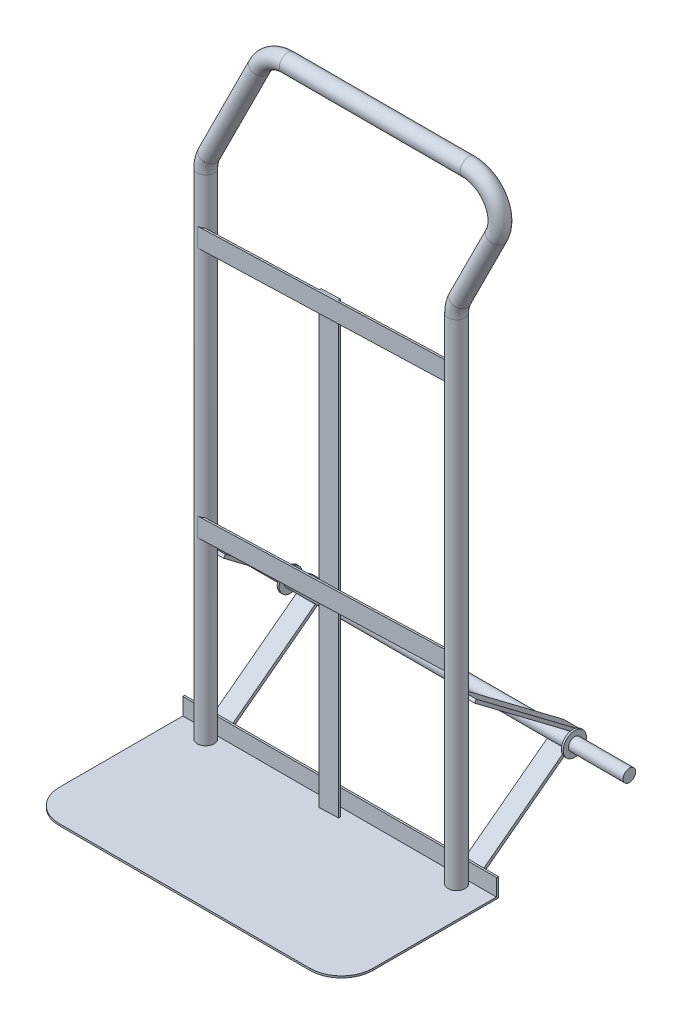
SolidWorks part; units mm, degrees
material "Plain Carbon Steel"
ref_plane "Front Plane" through (0, 0, 0) normal (0, 0, 1) x (1, 0, 0)
ref_plane "Top Plane" through (0, 0, 0) normal (0, 1, 0) x (1, 0, 0)
ref_plane "Right Plane" through (0, 0, 0) normal (1, 0, 0) x (0, 0, -1)
sketch3d "Frame Tube Path 3D Sketch"
  line L0 (0, 0, 0) -> (0, 788.1943, 0)
  line L1 (5.2806, 810.5589, 0) -> (63.8241, 927.6207, 0)
  line L2 (19.1047, 999.9853, 0) -> (-269.0871, 999.9853, 0)
  line L3 (-313.8065, 972.3498, 0) -> (-394.7194, 810.5589, 0)
  line L4 (-400, 788.1943, 0) -> (-400, 0, 0)
  arc A0 (0, 788.1943, 0) -> (5.2806, 810.5589, 0) centre (50, 788.1943, 0) ccw
  arc A1 (63.8241, 927.6207, 0) -> (19.1047, 999.9853, 0) centre (19.1047, 949.9853, 0) ccw
  arc A2 (-269.0871, 999.9853, 0) -> (-313.8065, 972.3498, 0) centre (-269.0871, 949.9853, 0) ccw
  arc A3 (-394.7194, 810.5589, 0) -> (-400, 788.1943, 0) centre (-350, 788.1943, 0) ccw
  point P9 (0, 800, 0)
  point P10 (50, 788.1943, -50)
  point P13 (100.0142, 999.9853, 0)
  point P14 (19.1047, 949.9853, 50)
  point P17 (-299.9858, 999.9853, 0)
  point P18 (-269.0871, 949.9853, 50)
  point P21 (-400, 800, 0)
  point P22 (-350, 788.1943, 50)
  dimension "D8" = 50
  dimension "D1" = 800
  dimension "D2" = 800
  dimension "D3" = 400
  dimension "D4" = 223.6
  dimension "D5" = 223.6
  dimension "D6" = 153.43
  dimension "D7" = 153.43
  dimension "D9" = 63.43
  dimension "D10" = 116.57
other "Pipe 26.9 X 3.2(1)"
ref_plane "Plane1" through (0, 0, 0) normal (0, 1, 0) x (1, 0, 0)
sketch "Sketch1" plane through (0, 0, 0) normal (0, 1, 0) x (1, 0, 0)
  circle A0 centre (0, 0) radius 10.25
  circle A1 centre (0, 0) radius 13.45
  point P3 (0, 13.45)
  point P5 (-13.45, 0)
  point P6 (0, -13.45)
  point P7 (13.45, 0)
  point P8 (0, 0)
  dimension "In_dia" = 20.5
  dimension "Out_dia" = 26.9
ref_plane "Plane2" through (0, 0, 0) normal (0.0336, 0, 0.9994) x (0.9994, 0, -0.0336)
sketch "Cross Bars Sketch" plane through (0, 0, 0) normal (0.0336, 0, 0.9994) x (0.9994, 0, -0.0336)
  line L0 (0, 0) -> (-399.7738, 0) construction
  line L1 (-199.8869, 0) -> (-199.8869, 957.4445) construction
  line L3 (0.1131, 715) -> (-399.8869, 715)
  line L4 (0.1131, 715) -> (0.1131, 685)
  line L5 (0.1131, 685) -> (-399.8869, 685)
  line L6 (-399.8869, 715) -> (-399.8869, 685)
  line L7 (0.1131, 715) -> (-399.8869, 685) construction
  line L8 (0.1131, 685) -> (-399.8869, 715) construction
  line L9 (0.1131, 315) -> (-399.8869, 315)
  line L10 (0.1131, 315) -> (0.1131, 285)
  line L11 (0.1131, 285) -> (-399.8869, 285)
  line L12 (-399.8869, 315) -> (-399.8869, 285)
  line L13 (0.1131, 315) -> (-399.8869, 285) construction
  line L14 (0.1131, 285) -> (-399.8869, 315) construction
  point P6 (-199.8869, 700)
  point P11 (-199.8869, 300)
  dimension "D1" = 30
  dimension "D2" = 400
  dimension "D3" = 30
  dimension "D4" = 400
  dimension "D5" = 370
  dimension "D6" = 715
extrude "Cross Bars 30x3" add sketch "Cross Bars Sketch" against normal blind 3 separate body
sketch "Centre Upright Sketch" plane through (-0.1009, 0, -2.9983) normal (-0.0336, 0, -0.9994) x (-0.9994, 0, 0.0336)
  line L0 (199.8869, 0) -> (199.8869, 715) construction
  line L2 (-0.1131, 315) -> (399.8869, 315) construction
  line L3 (-0.1131, 715) -> (399.8869, 715) construction
  line L5 (184.8869, 0) -> (214.8869, 0)
  line L6 (184.8869, 0) -> (184.8869, 715)
  line L7 (184.8869, 715) -> (214.8869, 715)
  line L8 (214.8869, 0) -> (214.8869, 715)
  line L9 (184.8869, 0) -> (214.8869, 715) construction
  line L10 (184.8869, 715) -> (214.8869, 0) construction
  point P4 (199.8869, 357.5)
  dimension "D1" = 30
  dimension "D2" = 42.5
extrude "Centre Upright Bar 30x3" add sketch "Centre Upright Sketch" along normal blind 3 separate body
ref_plane "Plane4" through (-200, 0, 0) normal (1, 0, 0) x (0, 0, -1)
sketch "Nose Plate Profile" plane through (-200, 0, 0) normal (1, 0, 0) x (0, 0, -1)
  line L0 (16.45, 27) -> (16.45, -3)
  line L1 (16.45, -3) -> (-233.55, -3)
  line L2 (-13.45, 0) -> (13.45, 0) construction
  line L3 (13.45, 0) -> (13.45, 788.1943) construction
  line L4 (13.45, 27) -> (13.45, 0)
  line L5 (13.45, 0) -> (-233.55, 0)
  line L6 (13.45, 27) -> (16.45, 27)
  line L7 (-233.55, 0) -> (-233.55, -3)
  dimension "D1" = 30
  dimension "D2" = 3
  dimension "D3" = 250
  dimension "D4" = 3
  dimension "D5" = 3
extrude "Nose Plate" add sketch "Nose Plate Profile" along normal mid plane 500 separate body
fillet "Nose Plate Corner Fillets R50" radius 50 2 edges at (-450, -1.5, 233.55) (50, -1.5, 233.55)
sketch "Axle Sketch Ø20" plane through (-200, 0, 0) normal (1, 0, 0) x (0, 0, -1)
  line L0 (-183.55, -3) -> (16.45, -3) construction
  line L1 (16.45, -3) -> (16.45, 27) construction
  circle A0 centre (160.45, 127) radius 10
  dimension "D1" = 20
  dimension "D2" = 130
  dimension "D3" = 144
extrude "Axle Ø20" add sketch "Axle Sketch Ø20" along normal mid plane 630 separate body
ref_plane "Plane5" through (0, 0, 0) normal (1, 0, 0) x (0, 0, -1)
sketch "Axle Bracket Profile" plane through (0, 0, 0) normal (1, 0, 0) x (0, 0, -1)
  line L0 (160.45, 127) -> (260.3131, 127) construction
  line L1 (160.45, 127) -> (12.5003, 127) construction
  line L2 (177.0664, 127) -> (13.45, 250.2938)
  line L3 (13.45, 0) -> (13.45, 788.1943) construction
  line L4 (177.0664, 127) -> (13.45, 3.7062)
  line L5 (185.3746, 127) -> (16.4591, 254.287)
  line L6 (185.3746, 127) -> (16.4591, -0.287)
  line L7 (13.45, 3.7062) -> (16.4591, -0.287)
  line L8 (13.45, 250.2938) -> (16.4591, 254.287)
  circle A0 centre (160.45, 127) radius 10 construction
  dimension "D1" = 37
  dimension "D2" = 5
extrude "Axle Bracket" add sketch "Axle Bracket Profile" along normal mid plane 30 separate body
mirror "Axle Bracket Mirror" about plane through (-200, 0, 0) normal (1, 0, 0) of "Axle Bracket"
ref_plane "Plane6" through (25, 0, 0) normal (1, 0, 0) x (0, 0, -1)
sketch "Wheel Collar Sketch Ø37" plane through (25, 0, 0) normal (1, 0, 0) x (0, 0, -1)
  circle A0 centre (160.45, 127) radius 18.5
  dimension "D1" = 37
extrude "Wheel Collar Ø37" add sketch "Wheel Collar Sketch Ø37" along normal blind 3 separate body
mirror "Wheel Collar Mirror" about plane through (-200, 0, 0) normal (1, 0, 0) of "Wheel Collar Ø37"
ref_plane "Plane8" through (-5.7499, 0, -170.9033) normal (0.0336, 0, 0.9994) x (0.9994, 0, -0.0336)
